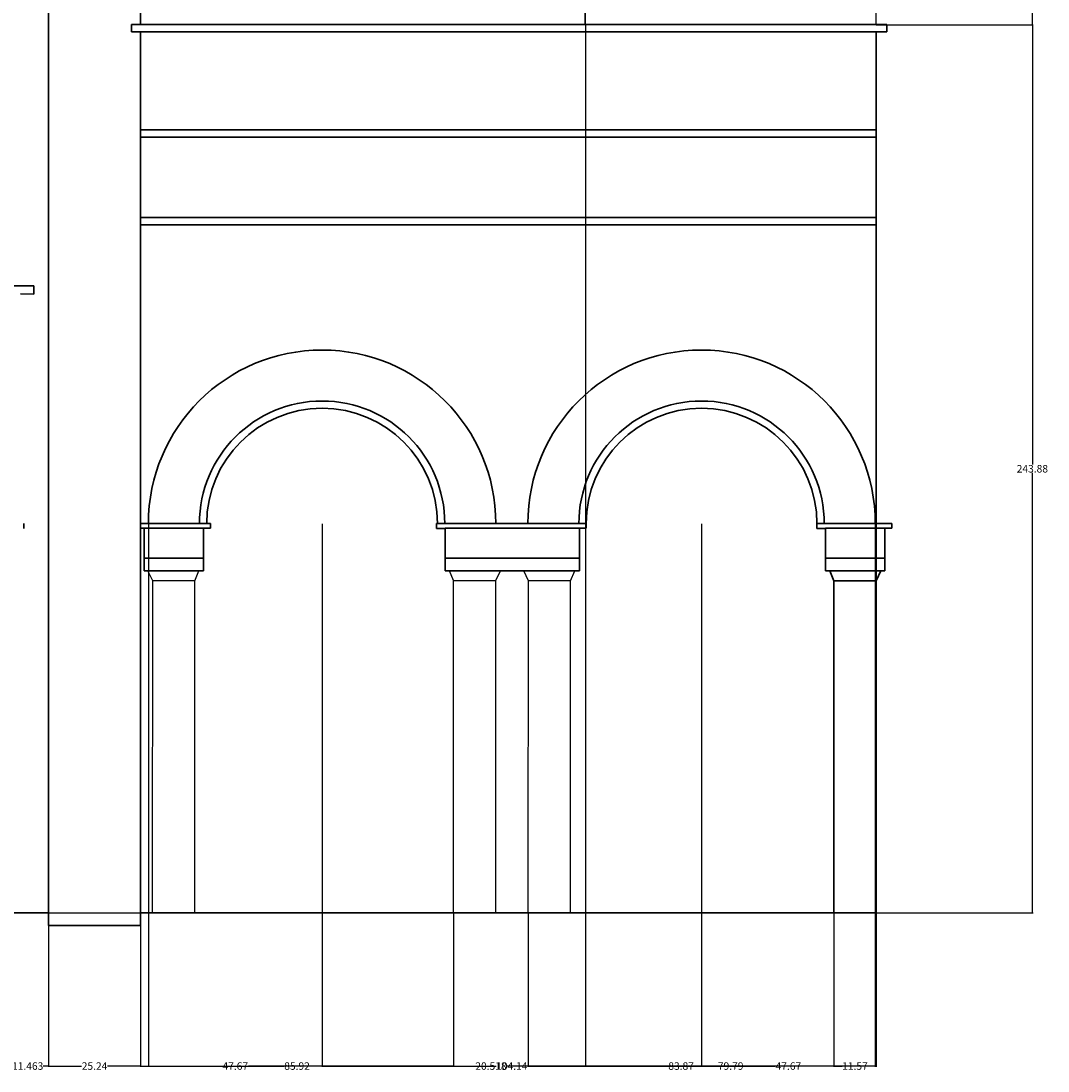
# Model space of a CAD drawing. Units: inches. Extents: x 14 to 859, y 52 to 711.
# Tile 10 of 11: x 577 to 859, y 52 to 341. Entities that reach past the tile are written whole.
import ezdxf

# ---------------------------------------------------------------- set-up
doc = ezdxf.new("R2010")
doc.units = ezdxf.units.IN
doc.header["$MEASUREMENT"] = 0
for name, color, linetype, lineweight in [('A-ANNO-DIMS', 2, 'Continuous', 18), ('A-COLS', 7, 'Continuous', 25), ('A-ELEV', 7, 'Continuous', 35)]:
    doc.layers.add(name, color=color, linetype=linetype, lineweight=lineweight)
doc.styles.get("Standard").update_dxf_attribs({"font": 'arial.ttf'})
doc.dimstyles.get("Standard").update_dxf_attribs({"dimtxt": 2.0625, "dimasz": 0.18, "dimexe": 0.18, "dimexo": 0.0625, "dimgap": 0.09, "dimtad": 0, "dimtih": 1, "dimtoh": 1, "dimdec": 4, "dimzin": 0, "dimdsep": 46, "dimlunit": 4, "dimtxsty": 'Standard', "dimcen": 0.09, "dimadec": 0, "dimazin": 0, "dimtfac": 1, "dimtdec": 4, "dimtofl": 0, "dimtmove": 0, "dimatfit": 3, "dimfxl": 1, "dimtolj": 1, "dimtzin": 0, "dimarcsym": 0})

# ---------------------------------------------------------------- blocks, each defined once
blk = doc.blocks.new('COLUMN')
for p, q in [((1.31, 91.21), (0, 93.94)), ((12.88, 91.21), (13.98, 93.94)), ((1.31, 0), (1.31, 91.21)), ((12.88, 91.21), (1.31, 91.21)), ((12.88, 0), (12.88, 91.21))]:
    blk.add_line(p, q)
blk = doc.blocks.new('*D13')
at = {"layer": 'A-ANNO-DIMS', "color": 0, "lineweight": -2, "transparency": 16777216}
for p, q in [((60.78, 339.73), (60.78, 709.71)), ((60.96, 709.53), (432.6, 709.53)), ((811.37, 709.53), (439.73, 709.53)), ((811.55, 339.73), (811.55, 709.71))]:
    blk.add_line(p, q, dxfattribs=at)
at = {"layer": 'A-ANNO-DIMS', "color": 0, "transparency": 16777216}
for points in [[(60.96, 709.56), (60.96, 709.5), (60.78, 709.53)], [(811.37, 709.56), (811.37, 709.5), (811.55, 709.53)]]:
    blk.add_solid(points, dxfattribs=at)
at = {"layer": 'Defpoints', "color": 0, "transparency": 16777216}
for p in [(811.55, 709.53), (60.78, 339.66), (811.55, 339.66)]:
    blk.add_point(p, dxfattribs=at)
at = {"layer": 'A-ANNO-DIMS', "color": 0, "transparency": 16777216, "insert": (436.17, 709.53), "char_height": 2.062, "attachment_point": 5}
blk.add_mtext('\\A1;750.8', dxfattribs=at)
blk = doc.blocks.new('*D15')
at = {"layer": 'A-ANNO-DIMS', "color": 0, "lineweight": -2, "transparency": 16777216}
for p, q in [((584.44, 92.27), (584.44, 53.56)), ((609.68, 92.27), (609.68, 53.56)), ((584.62, 53.74), (593.48, 53.74)), ((609.5, 53.74), (600.64, 53.74))]:
    blk.add_line(p, q, dxfattribs=at)
at = {"layer": 'A-ANNO-DIMS', "color": 0, "transparency": 16777216}
for points in [[(584.62, 53.77), (584.62, 53.71), (584.44, 53.74)], [(609.5, 53.77), (609.5, 53.71), (609.68, 53.74)]]:
    blk.add_solid(points, dxfattribs=at)
at = {"layer": 'Defpoints', "color": 0, "transparency": 16777216}
for p in [(584.44, 92.34), (609.68, 92.34), (609.68, 53.74)]:
    blk.add_point(p, dxfattribs=at)
at = {"layer": 'A-ANNO-DIMS', "color": 0, "transparency": 16777216, "insert": (597.06, 53.74), "char_height": 2.062, "attachment_point": 5}
blk.add_mtext('\\A1;25.24', dxfattribs=at)
blk = doc.blocks.new('*D17')
at = {"layer": 'A-ANNO-DIMS', "color": 0, "lineweight": -2, "transparency": 16777216}
for p, q in [((811.62, 339.66), (854.64, 339.66)), ((854.46, 339.48), (854.46, 218.87)), ((854.46, 95.97), (854.46, 216.58)), ((584.5, 95.79), (854.64, 95.79))]:
    blk.add_line(p, q, dxfattribs=at)
at = {"layer": 'A-ANNO-DIMS', "color": 0, "transparency": 16777216}
for points in [[(854.43, 339.48), (854.49, 339.48), (854.46, 339.66)], [(854.43, 95.97), (854.49, 95.97), (854.46, 95.79)]]:
    blk.add_solid(points, dxfattribs=at)
at = {"layer": 'Defpoints', "color": 0, "transparency": 16777216}
for p in [(811.55, 339.66), (854.46, 339.66), (584.44, 95.79)]:
    blk.add_point(p, dxfattribs=at)
at = {"layer": 'A-ANNO-DIMS', "color": 0, "transparency": 16777216, "insert": (854.46, 217.73), "char_height": 2.062, "attachment_point": 5}
blk.add_mtext('\\A1;243.88', dxfattribs=at)
blk = doc.blocks.new('*D18')
at = {"layer": 'A-ANNO-DIMS', "color": 0, "lineweight": -2, "transparency": 16777216}
for p, q in [((584.68, 404.37), (854.64, 404.37)), ((854.46, 404.19), (854.46, 373.16)), ((854.46, 339.84), (854.46, 370.87)), ((811.62, 339.66), (854.64, 339.66))]:
    blk.add_line(p, q, dxfattribs=at)
at = {"layer": 'A-ANNO-DIMS', "color": 0, "transparency": 16777216}
for points in [[(854.43, 404.19), (854.49, 404.19), (854.46, 404.37)], [(854.43, 339.84), (854.49, 339.84), (854.46, 339.66)]]:
    blk.add_solid(points, dxfattribs=at)
at = {"layer": 'Defpoints', "color": 0, "transparency": 16777216}
for p in [(584.62, 404.37), (854.46, 404.37), (811.55, 339.66)]:
    blk.add_point(p, dxfattribs=at)
at = {"layer": 'A-ANNO-DIMS', "color": 0, "transparency": 16777216, "insert": (854.46, 372.02), "char_height": 2.062, "attachment_point": 5}
blk.add_mtext('\\A1;64.71', dxfattribs=at)
blk = doc.blocks.new('*D34')
at = {"layer": 'A-ANNO-DIMS', "color": 0, "lineweight": -2, "transparency": 16777216}
for p, q in [((572.98, 95.73), (572.98, 53.56)), ((584.44, 95.73), (584.44, 53.56)), ((573.16, 53.74), (574.44, 53.74)), ((584.26, 53.74), (582.98, 53.74))]:
    blk.add_line(p, q, dxfattribs=at)
at = {"layer": 'A-ANNO-DIMS', "color": 0, "transparency": 16777216}
for points in [[(573.16, 53.77), (573.16, 53.71), (572.98, 53.74)], [(584.26, 53.77), (584.26, 53.71), (584.44, 53.74)]]:
    blk.add_solid(points, dxfattribs=at)
at = {"layer": 'Defpoints', "color": 0, "transparency": 16777216}
for p in [(572.98, 95.79), (584.44, 95.79), (584.44, 53.74)]:
    blk.add_point(p, dxfattribs=at)
at = {"layer": 'A-ANNO-DIMS', "color": 0, "transparency": 16777216, "insert": (578.71, 53.74), "char_height": 2.062, "attachment_point": 5}
blk.add_mtext('\\A1;11.463', dxfattribs=at)
blk = doc.blocks.new('*D73')
at = {"layer": 'A-ANNO-DIMS', "color": 0, "lineweight": -2, "transparency": 16777216}
for p, q in [((611.85, 202.6), (611.85, 53.56)), ((659.52, 202.6), (659.52, 53.56)), ((612.03, 53.74), (632.07, 53.74)), ((659.34, 53.74), (639.3, 53.74))]:
    blk.add_line(p, q, dxfattribs=at)
at = {"layer": 'A-ANNO-DIMS', "color": 0, "transparency": 16777216}
for points in [[(612.03, 53.77), (612.03, 53.71), (611.85, 53.74)], [(659.34, 53.77), (659.34, 53.71), (659.52, 53.74)]]:
    blk.add_solid(points, dxfattribs=at)
at = {"layer": 'Defpoints', "color": 0, "transparency": 16777216}
for p in [(611.85, 202.66), (659.52, 202.66), (659.52, 53.74)]:
    blk.add_point(p, dxfattribs=at)
at = {"layer": 'A-ANNO-DIMS', "color": 0, "transparency": 16777216, "insert": (635.69, 53.74), "char_height": 2.062, "attachment_point": 5}
blk.add_mtext('\\A1;47.67', dxfattribs=at)
blk = doc.blocks.new('*D74')
at = {"layer": 'A-ANNO-DIMS', "color": 0, "lineweight": -2, "transparency": 16777216}
for p, q in [((659.52, 202.6), (659.52, 53.56)), ((763.66, 202.6), (763.66, 53.56)), ((659.7, 53.74), (707.32, 53.74)), ((763.48, 53.74), (715.86, 53.74))]:
    blk.add_line(p, q, dxfattribs=at)
at = {"layer": 'A-ANNO-DIMS', "color": 0, "transparency": 16777216}
for points in [[(659.7, 53.77), (659.7, 53.71), (659.52, 53.74)], [(763.48, 53.77), (763.48, 53.71), (763.66, 53.74)]]:
    blk.add_solid(points, dxfattribs=at)
at = {"layer": 'Defpoints', "color": 0, "transparency": 16777216}
for p in [(659.52, 202.66), (763.66, 202.66), (763.66, 53.74)]:
    blk.add_point(p, dxfattribs=at)
at = {"layer": 'A-ANNO-DIMS', "color": 0, "transparency": 16777216, "insert": (711.59, 53.74), "char_height": 2.062, "attachment_point": 5}
blk.add_mtext('\\A1;104.14', dxfattribs=at)
blk = doc.blocks.new('*D75')
at = {"layer": 'A-ANNO-DIMS', "color": 0, "lineweight": -2, "transparency": 16777216}
for p, q in [((763.66, 202.6), (763.66, 53.56)), ((811.34, 202.6), (811.34, 53.56)), ((763.84, 53.74), (783.89, 53.74)), ((811.16, 53.74), (791.11, 53.74))]:
    blk.add_line(p, q, dxfattribs=at)
at = {"layer": 'A-ANNO-DIMS', "color": 0, "transparency": 16777216}
for points in [[(763.84, 53.77), (763.84, 53.71), (763.66, 53.74)], [(811.16, 53.77), (811.16, 53.71), (811.34, 53.74)]]:
    blk.add_solid(points, dxfattribs=at)
at = {"layer": 'Defpoints', "color": 0, "transparency": 16777216}
for p in [(763.66, 202.66), (811.34, 202.66), (811.34, 53.74)]:
    blk.add_point(p, dxfattribs=at)
at = {"layer": 'A-ANNO-DIMS', "color": 0, "transparency": 16777216, "insert": (787.5, 53.74), "char_height": 2.062, "attachment_point": 5}
blk.add_mtext('\\A1;47.67', dxfattribs=at)
blk = doc.blocks.new('*D76')
at = {"layer": 'A-ANNO-DIMS', "color": 0, "lineweight": -2, "transparency": 16777216}
for p, q in [((609.68, 95.73), (609.68, 53.56)), ((695.6, 95.74), (695.6, 53.56)), ((609.86, 53.74), (649.08, 53.74)), ((695.42, 53.74), (656.2, 53.74))]:
    blk.add_line(p, q, dxfattribs=at)
at = {"layer": 'A-ANNO-DIMS', "color": 0, "transparency": 16777216}
for points in [[(609.86, 53.77), (609.86, 53.71), (609.68, 53.74)], [(695.42, 53.77), (695.42, 53.71), (695.6, 53.74)]]:
    blk.add_solid(points, dxfattribs=at)
at = {"layer": 'Defpoints', "color": 0, "transparency": 16777216}
for p in [(609.68, 95.79), (695.6, 95.8), (695.6, 53.74)]:
    blk.add_point(p, dxfattribs=at)
at = {"layer": 'A-ANNO-DIMS', "color": 0, "transparency": 16777216, "insert": (652.64, 53.74), "char_height": 2.062, "attachment_point": 5}
blk.add_mtext('\\A1;85.92', dxfattribs=at)
blk = doc.blocks.new('*D77')
at = {"layer": 'A-ANNO-DIMS', "color": 0, "lineweight": -2, "transparency": 16777216}
for p, q in [((695.6, 95.74), (695.6, 53.56)), ((716.12, 95.73), (716.12, 53.56)), ((695.78, 53.74), (701.47, 53.74)), ((715.94, 53.74), (710.25, 53.74))]:
    blk.add_line(p, q, dxfattribs=at)
at = {"layer": 'A-ANNO-DIMS', "color": 0, "transparency": 16777216}
for points in [[(695.78, 53.77), (695.78, 53.71), (695.6, 53.74)], [(715.94, 53.77), (715.94, 53.71), (716.12, 53.74)]]:
    blk.add_solid(points, dxfattribs=at)
at = {"layer": 'Defpoints', "color": 0, "transparency": 16777216}
for p in [(695.6, 95.8), (716.12, 95.79), (716.12, 53.74)]:
    blk.add_point(p, dxfattribs=at)
at = {"layer": 'A-ANNO-DIMS', "color": 0, "transparency": 16777216, "insert": (705.86, 53.74), "char_height": 2.062, "attachment_point": 5}
blk.add_mtext('\\A1;20.518', dxfattribs=at)
blk = doc.blocks.new('*D78')
at = {"layer": 'A-ANNO-DIMS', "color": 0, "lineweight": -2, "transparency": 16777216}
for p, q in [((716.12, 95.73), (716.12, 53.56)), ((799.98, 95.73), (799.98, 53.56)), ((716.3, 53.74), (754.48, 53.74)), ((799.8, 53.74), (761.62, 53.74))]:
    blk.add_line(p, q, dxfattribs=at)
at = {"layer": 'A-ANNO-DIMS', "color": 0, "transparency": 16777216}
for points in [[(716.3, 53.77), (716.3, 53.71), (716.12, 53.74)], [(799.8, 53.77), (799.8, 53.71), (799.98, 53.74)]]:
    blk.add_solid(points, dxfattribs=at)
at = {"layer": 'Defpoints', "color": 0, "transparency": 16777216}
for p in [(716.12, 95.79), (799.98, 95.79), (799.98, 53.74)]:
    blk.add_point(p, dxfattribs=at)
at = {"layer": 'A-ANNO-DIMS', "color": 0, "transparency": 16777216, "insert": (758.05, 53.74), "char_height": 2.062, "attachment_point": 5}
blk.add_mtext('\\A1;83.87', dxfattribs=at)
blk = doc.blocks.new('*D79')
at = {"layer": 'A-ANNO-DIMS', "color": 0, "lineweight": -2, "transparency": 16777216}
for p, q in [((799.98, 95.73), (799.98, 53.56)), ((811.55, 95.73), (811.55, 53.56)), ((800.16, 53.74), (802.3, 53.74)), ((811.37, 53.74), (809.24, 53.74))]:
    blk.add_line(p, q, dxfattribs=at)
at = {"layer": 'A-ANNO-DIMS', "color": 0, "transparency": 16777216}
for points in [[(800.16, 53.77), (800.16, 53.71), (799.98, 53.74)], [(811.37, 53.77), (811.37, 53.71), (811.55, 53.74)]]:
    blk.add_solid(points, dxfattribs=at)
at = {"layer": 'Defpoints', "color": 0, "transparency": 16777216}
for p in [(799.98, 95.79), (811.55, 95.79), (811.55, 53.74)]:
    blk.add_point(p, dxfattribs=at)
at = {"layer": 'A-ANNO-DIMS', "color": 0, "transparency": 16777216, "insert": (805.77, 53.74), "char_height": 2.062, "attachment_point": 5}
blk.add_mtext('\\A1;11.57', dxfattribs=at)
blk = doc.blocks.new('*D85')
at = {"layer": 'A-ANNO-DIMS', "color": 0, "lineweight": -2, "transparency": 16777216}
for p, q in [((731.77, 339.6), (731.77, 53.56)), ((811.55, 337.6), (811.55, 53.56)), ((731.95, 53.74), (768.1, 53.74)), ((811.37, 53.74), (775.22, 53.74))]:
    blk.add_line(p, q, dxfattribs=at)
at = {"layer": 'A-ANNO-DIMS', "color": 0, "transparency": 16777216}
for points in [[(731.95, 53.77), (731.95, 53.71), (731.77, 53.74)], [(811.37, 53.77), (811.37, 53.71), (811.55, 53.74)]]:
    blk.add_solid(points, dxfattribs=at)
at = {"layer": 'Defpoints', "color": 0, "transparency": 16777216}
for p in [(731.77, 339.66), (811.55, 337.66), (811.55, 53.74)]:
    blk.add_point(p, dxfattribs=at)
at = {"layer": 'A-ANNO-DIMS', "color": 0, "transparency": 16777216, "insert": (771.66, 53.74), "char_height": 2.062, "attachment_point": 5}
blk.add_mtext('\\A1;79.79', dxfattribs=at)

msp = doc.modelspace()

# ---------------------------------------------------------------- linework, layer by layer
at = {"layer": 'A-ELEV'}
for p, q in [((731.7655, 339.6626), (731.7655, 404.3712)), ((584.4409, 304.6217), (584.4409, 371.6812)), ((609.6802, 339.6626), (609.6802, 370.2389)), ((609.6802, 339.6626), (607.2115, 339.6626)), ((607.2115, 339.6626), (607.2115, 337.6626)), ((607.2115, 337.6626), (609.6802, 337.6626)), ((811.5534, 339.6626), (609.6802, 339.6626)), ((609.6802, 302.6), (609.6802, 337.6626)), ((811.5534, 337.6626), (609.6802, 337.6626)), ((811.5534, 339.6626), (814.5179, 339.6626)), ((811.5534, 303.3146), (811.5534, 337.6626)), ((814.5179, 337.6626), (811.5534, 337.6626)), ((814.5179, 339.6626), (814.5179, 337.6626)), ((811.5534, 310.8171), (609.6802, 310.8171)), ((811.5534, 308.8171), (609.6802, 308.8171)), ((584.4409, 92.3364), (584.4409, 304.6217)), ((811.5534, 263.7876), (811.5534, 303.3146)), ((609.6802, 202.6598), (609.6802, 302.6)), ((811.5534, 286.7316), (609.6802, 286.7316)), ((811.5534, 284.7316), (609.6802, 284.7316)), ((503.2589, 267.9895), (580.3801, 267.9895)), ((580.3801, 265.6361), (576.7277, 265.7663)), ((580.3801, 267.9895), (580.3801, 265.6361)), ((811.5534, 202.6598), (811.5534, 263.7876)), ((577.6252, 202.6598), (577.6252, 201.3212)), ((628.8481, 202.6598), (609.6802, 202.6598)), ((609.6802, 202.6598), (609.6802, 92.3364)), ((628.8481, 201.4021), (628.8481, 202.6598)), ((711.4693, 202.6598), (690.9504, 202.6598)), ((690.9504, 202.6598), (690.9504, 201.3212)), ((731.9882, 202.6598), (711.4693, 202.6598)), ((731.9882, 201.4021), (731.9882, 202.6598)), ((815.8554, 202.6598), (795.3365, 202.6598)), ((795.3365, 202.6598), (795.3365, 201.3212)), ((815.8554, 201.4021), (815.8554, 202.6598)), ((609.6802, 201.4021), (610.6465, 201.4021)), ((626.9914, 201.4021), (610.6465, 201.4021)), ((610.6465, 201.4021), (610.6465, 193.2091)), ((626.9914, 193.2091), (626.9914, 201.4021)), ((626.9914, 201.4021), (628.8481, 201.4021)), ((690.9504, 201.3212), (693.2677, 201.3212)), ((709.6126, 201.4021), (693.2677, 201.4021)), ((693.2677, 201.4021), (693.2677, 193.2091)), ((709.6126, 201.4021), (711.4693, 201.4021)), ((713.7866, 201.4021), (711.4693, 201.4021)), ((730.1315, 201.4021), (713.7866, 201.4021)), ((730.1315, 193.2091), (730.1315, 201.4021)), ((730.1315, 201.4021), (731.9882, 201.4021)), ((795.3365, 201.3212), (797.6538, 201.3212)), ((813.9987, 201.4021), (797.6538, 201.4021)), ((797.6538, 201.4021), (797.6538, 193.2091)), ((813.9987, 193.2091), (813.9987, 201.4021)), ((813.9987, 201.4021), (815.8554, 201.4021)), ((626.9914, 193.2091), (610.6465, 193.2091)), ((610.6465, 193.2091), (610.6465, 189.7289)), ((626.9914, 189.7289), (626.9914, 193.2091)), ((709.6126, 193.2091), (693.2677, 193.2091)), ((693.2677, 193.2091), (693.2677, 189.7289)), ((713.7866, 193.2091), (709.6126, 193.2091)), ((730.1315, 193.2091), (713.7866, 193.2091)), ((730.1315, 189.7289), (730.1315, 193.2091)), ((813.9987, 193.2091), (797.6538, 193.2091)), ((797.6538, 193.2091), (797.6538, 189.7289)), ((813.9987, 189.7289), (813.9987, 193.2091)), ((610.6465, 189.7289), (626.9914, 189.7289)), ((693.2677, 189.7289), (709.6126, 189.7289)), ((713.7866, 189.7289), (709.6126, 189.7289)), ((713.7866, 189.7289), (730.1315, 189.7289)), ((797.6538, 189.7289), (813.9987, 189.7289)), ((799.9838, 187.0003), (798.8775, 189.7289)), ((811.5534, 187.0003), (812.8613, 189.7289)), ((799.9838, 95.7876), (799.9838, 187.0003)), ((799.9838, 187.0003), (811.5534, 187.0003)), ((811.5534, 95.7876), (811.5534, 187.0003)), ((287.893, 95.7876), (584.4409, 95.7876)), ((609.6802, 95.7876), (811.5534, 95.7876)), ((609.6802, 92.3364), (584.4409, 92.3364))]:
    msp.add_line(p, q, dxfattribs=at)
for centre, radius in [((659.5231, 202.6598), 47.6742), ((763.6623, 202.6598), 47.6742), ((659.5231, 202.6598), 33.6742), ((659.5231, 202.6598), 31.6742), ((763.6623, 202.6598), 33.6742), ((763.6623, 202.6598), 31.6742)]:
    msp.add_arc(centre, radius, 0, 180, dxfattribs=at)

# ---------------------------------------------------------------- block references
at = {"layer": 'A-COLS', "rotation": 359.9687779280772}
for p in [(611.6691, 95.7919), (714.8092, 95.7919)]:
    msp.add_blockref('COLUMN', p, dxfattribs=at)
at = {"layer": 'A-COLS', "extrusion": (0, 0, -1), "zscale": -1, "rotation": 359.9990108211547}
msp.add_blockref('COLUMN', (-708.4762, 95.8043), dxfattribs=at)

# ---------------------------------------------------------------- dimensions: what is measured, and where the dimension line sits
at = {"layer": 'A-ANNO-DIMS'}
for base, p1, p2, override, picture, middle in [((811.5534, 709.5262), (60.7804, 339.6626), (811.5534, 339.6626), {"dimdec": 1, "dimlfac": 1, "dimrnd": 0, "dimzin": 0, "dimdsep": 46, "dimlunit": 2}, '*D13', (436.1669, 709.5262)), ((811.5534, 53.7364), (731.7655, 339.6626), (811.5534, 337.6626), {"dimdec": 2, "dimlfac": 1, "dimrnd": 0, "dimzin": 0, "dimdsep": 46, "dimlunit": 2}, '*D85', (771.6595, 53.7364)), ((659.5231, 53.7364), (611.8489, 202.6598), (659.5231, 202.6598), {"dimdec": 2, "dimlfac": 1, "dimrnd": 0, "dimzin": 0, "dimdsep": 46, "dimlunit": 2}, '*D73', (635.686, 53.7364)), ((763.6623, 53.7364), (659.5231, 202.6598), (763.6623, 202.6598), {"dimdec": 2, "dimlfac": 1, "dimrnd": 0, "dimzin": 0, "dimdsep": 46, "dimlunit": 2}, '*D74', (711.5927, 53.7364)), ((811.3365, 53.7364), (763.6623, 202.6598), (811.3365, 202.6598), {"dimdec": 2, "dimlfac": 1, "dimrnd": 0, "dimzin": 0, "dimdsep": 46, "dimlunit": 2}, '*D75', (787.4994, 53.7364)), ((584.4409, 53.7364), (572.9779, 95.7876), (584.4409, 95.7876), {"dimdec": 3, "dimlfac": 1, "dimrnd": 0, "dimzin": 0, "dimdsep": 46, "dimlunit": 2}, '*D34', (578.7094, 53.7364)), ((695.5989, 53.7364), (609.6802, 95.7876), (695.5989, 95.8037), {"dimdec": 2, "dimlfac": 1, "dimrnd": 0, "dimzin": 0, "dimdsep": 46, "dimlunit": 2}, '*D76', (652.6396, 53.7364)), ((716.1168, 53.7364), (695.5989, 95.8037), (716.1168, 95.7908), {"dimdec": 3, "dimlfac": 1, "dimrnd": 0, "dimzin": 0, "dimdsep": 46, "dimlunit": 2}, '*D77', (705.8579, 53.7364)), ((799.9838, 53.7364), (716.1168, 95.7908), (799.9838, 95.7876), {"dimdec": 2, "dimlfac": 1, "dimrnd": 0, "dimzin": 0, "dimdsep": 46, "dimlunit": 2}, '*D78', (758.0503, 53.7364)), ((811.5534, 53.7364), (799.9838, 95.7876), (811.5534, 95.7876), {"dimdec": 2, "dimlfac": 1, "dimrnd": 0, "dimzin": 0, "dimdsep": 46, "dimlunit": 2}, '*D79', (805.7686, 53.7364)), ((609.6802, 53.7364), (584.4409, 92.3364), (609.6802, 92.3364), {"dimdec": 2, "dimlfac": 1, "dimrnd": 0, "dimzin": 0, "dimdsep": 46, "dimlunit": 2}, '*D15', (597.0605, 53.7364))]:
    dim = msp.add_linear_dim(base=base, p1=p1, p2=p2, dimstyle='Standard', override=override, dxfattribs=at)
    dim.commit()
    dim.dimension.update_dxf_attribs({"geometry": picture, "text_midpoint": middle})
for base, p1, p2, picture, middle in [((854.4554, 404.3712), (811.5534, 339.6626), (584.619, 404.3712), '*D18', (854.4554, 372.0169)), ((854.45536, 339.66265), (584.44087, 95.78764), (811.55345, 339.66265), '*D17', (854.45536, 217.72514))]:
    dim = msp.add_linear_dim(base=base, p1=p1, p2=p2, angle=90, dimstyle='Standard', override={"dimdec": 2, "dimlfac": 1, "dimrnd": 0, "dimzin": 0, "dimdsep": 46, "dimlunit": 2}, dxfattribs=at)
    dim.commit()
    dim.dimension.update_dxf_attribs({"geometry": picture, "text_midpoint": middle})

doc.saveas('drawing.dxf')
